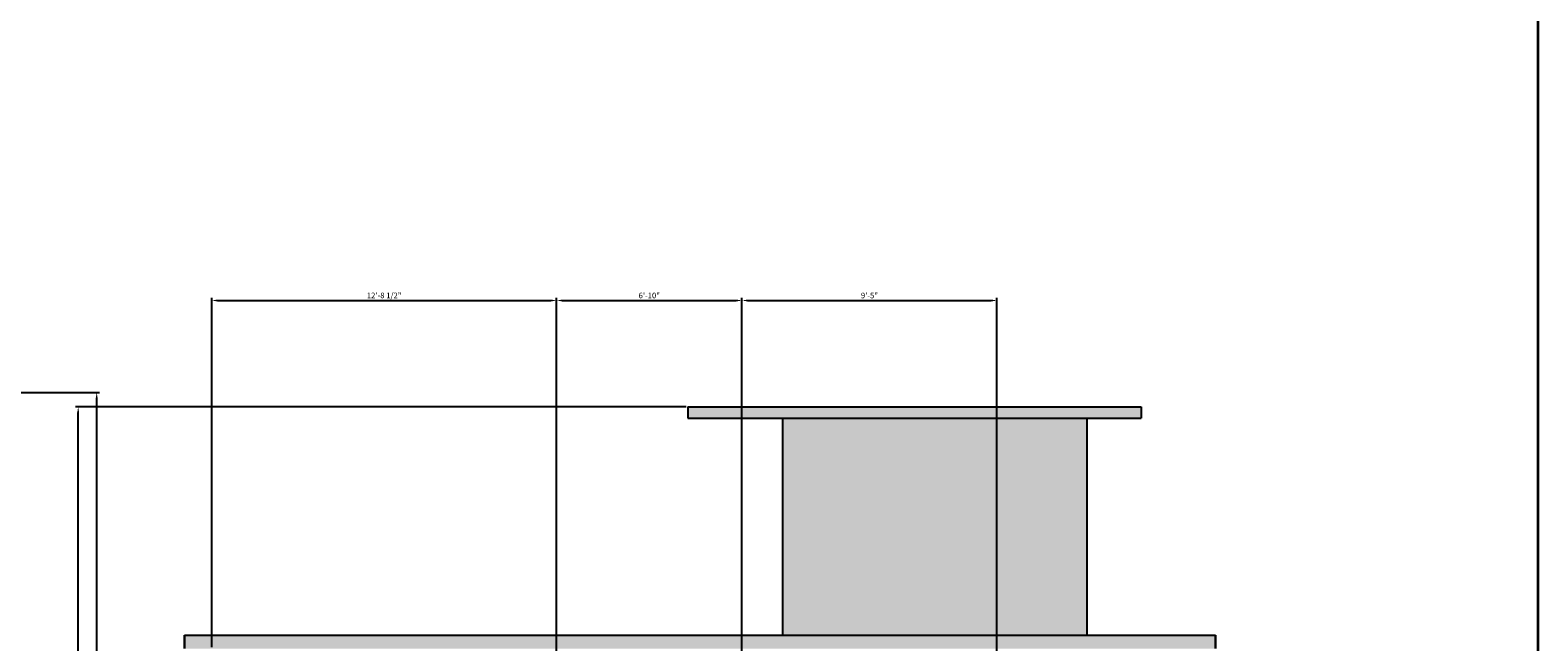
# Model space of a CAD drawing. Units: inches. Extents: x 2391 to 16591, y 7259 to 10239.
# Tile 16 of 27: x 3487 to 4154, y 8229 to 8500. Entities that reach past the tile are written whole.
import ezdxf

# ---------------------------------------------------------------- set-up
doc = ezdxf.new("R2010")
doc.units = ezdxf.units.IN
for name, color, linetype, lineweight in [('A-ANNO-DIMS', 4, 'Continuous', 18), ('A-ANNO-TTLB', 7, 'Continuous', 35), ('A-ELEV', 7, 'Continuous', 30), ('A-ELEV-SURF-PATT', 253, 'Continuous', 13), ('A-ROOF', 7, 'Continuous', 25)]:
    doc.layers.add(name, color=color, linetype=linetype, lineweight=lineweight)
doc.styles.get("Standard").update_dxf_attribs({"font": 'arial.ttf'})
doc.dimstyles.new('ISO-25', dxfattribs={"dimtxt": 2.5, "dimasz": 2.5, "dimexe": 1.25, "dimexo": 0.625, "dimtad": 1, "dimdec": 0, "dimlunit": 3, "dimtxsty": 'Standard', "dimcen": 2.5, "dimadec": 0, "dimazin": 0, "dimtfac": 1, "dimtdec": 0, "dimtmove": 0, "dimatfit": 3, "dimfxl": 1, "dimarcsym": 0})

# ---------------------------------------------------------------- blocks, each defined once
blk = doc.blocks.new('*D84')
at = {"layer": 'A-ANNO-DIMS', "color": 0, "lineweight": -2, "transparency": 16777216}
for p, q in [((3437.4, 8339.52), (3518.08, 8339.52)), ((3516.83, 7579.02), (3516.83, 8337.02)), ((3464.4, 7576.52), (3518.08, 7576.52))]:
    blk.add_line(p, q, dxfattribs=at)
at = {"layer": 'A-ANNO-DIMS', "color": 0, "transparency": 16777216}
for points in [[(3516.41, 8337.02), (3517.24, 8337.02), (3516.83, 8339.52)], [(3516.41, 7579.02), (3517.24, 7579.02), (3516.83, 7576.52)]]:
    blk.add_solid(points, dxfattribs=at)
at = {"layer": 'Defpoints', "color": 0, "transparency": 16777216}
for p in [(3436.78, 8339.52), (3516.83, 8339.52), (3463.78, 7576.52)]:
    blk.add_point(p, dxfattribs=at)
at = {"layer": 'A-ANNO-DIMS', "color": 0, "transparency": 16777216, "insert": (3514.93, 7958.02), "char_height": 2.5, "attachment_point": 5, "rotation": 90}
blk.add_mtext('63\'-7"', dxfattribs=at)
blk = doc.blocks.new('*D92')
at = {"layer": 'A-ANNO-DIMS', "color": 0, "lineweight": -2, "transparency": 16777216}
for p, q in [((3777.58, 8333.18), (3507.41, 8333.18)), ((3508.66, 7572.68), (3508.66, 8330.68)), ((3561.08, 7570.18), (3507.41, 7570.18))]:
    blk.add_line(p, q, dxfattribs=at)
at = {"layer": 'A-ANNO-DIMS', "color": 0, "transparency": 16777216}
for points in [[(3508.24, 8330.68), (3509.08, 8330.68), (3508.66, 8333.18)], [(3508.24, 7572.68), (3509.08, 7572.68), (3508.66, 7570.18)]]:
    blk.add_solid(points, dxfattribs=at)
at = {"layer": 'Defpoints', "color": 0, "transparency": 16777216}
for p in [(3508.66, 8333.18), (3778.21, 8333.18), (3561.71, 7570.18)]:
    blk.add_point(p, dxfattribs=at)
at = {"layer": 'A-ANNO-DIMS', "color": 0, "transparency": 16777216, "insert": (3506.76, 7951.68), "char_height": 2.5, "attachment_point": 5, "rotation": 90}
blk.add_mtext('63\'-7"', dxfattribs=at)
blk = doc.blocks.new('*D93')
at = {"layer": 'A-ANNO-DIMS', "color": 0, "lineweight": -2, "transparency": 16777216}
for p, q in [((3567.71, 8226.81), (3567.71, 8381.48)), ((3570.21, 8380.23), (3717.71, 8380.23)), ((3720.21, 8172.81), (3720.21, 8381.48))]:
    blk.add_line(p, q, dxfattribs=at)
at = {"layer": 'A-ANNO-DIMS', "color": 0, "transparency": 16777216}
for points in [[(3570.21, 8380.65), (3570.21, 8379.81), (3567.71, 8380.23)], [(3717.71, 8380.65), (3717.71, 8379.81), (3720.21, 8380.23)]]:
    blk.add_solid(points, dxfattribs=at)
at = {"layer": 'Defpoints', "color": 0, "transparency": 16777216}
for p in [(3720.21, 8380.23), (3567.71, 8226.18), (3720.21, 8172.18)]:
    blk.add_point(p, dxfattribs=at)
at = {"layer": 'A-ANNO-DIMS', "color": 0, "transparency": 16777216, "insert": (3643.96, 8382.15), "char_height": 2.5, "attachment_point": 5}
blk.add_mtext('12\'-8 1/2"', dxfattribs=at)
blk = doc.blocks.new('*D94')
at = {"layer": 'A-ANNO-DIMS', "color": 0, "lineweight": -2, "transparency": 16777216}
for p, q in [((3720.21, 8172.81), (3720.21, 8381.48)), ((3722.71, 8380.23), (3799.71, 8380.23)), ((3802.21, 8172.81), (3802.21, 8381.48))]:
    blk.add_line(p, q, dxfattribs=at)
at = {"layer": 'A-ANNO-DIMS', "color": 0, "transparency": 16777216}
for points in [[(3722.71, 8380.65), (3722.71, 8379.81), (3720.21, 8380.23)], [(3799.71, 8380.65), (3799.71, 8379.81), (3802.21, 8380.23)]]:
    blk.add_solid(points, dxfattribs=at)
at = {"layer": 'Defpoints', "color": 0, "transparency": 16777216}
for p in [(3802.21, 8380.23), (3720.21, 8172.18), (3802.21, 8172.18)]:
    blk.add_point(p, dxfattribs=at)
at = {"layer": 'A-ANNO-DIMS', "color": 0, "transparency": 16777216, "insert": (3761.21, 8382.13), "char_height": 2.5, "attachment_point": 5}
blk.add_mtext('6\'-10"', dxfattribs=at)
blk = doc.blocks.new('*D95')
at = {"layer": 'A-ANNO-DIMS', "color": 0, "lineweight": -2, "transparency": 16777216}
for p, q in [((3802.21, 8172.81), (3802.21, 8381.48)), ((3804.71, 8380.23), (3912.46, 8380.23)), ((3914.96, 8172.81), (3914.96, 8381.48))]:
    blk.add_line(p, q, dxfattribs=at)
at = {"layer": 'A-ANNO-DIMS', "color": 0, "transparency": 16777216}
for points in [[(3804.71, 8380.65), (3804.71, 8379.81), (3802.21, 8380.23)], [(3912.46, 8380.65), (3912.46, 8379.81), (3914.96, 8380.23)]]:
    blk.add_solid(points, dxfattribs=at)
at = {"layer": 'Defpoints', "color": 0, "transparency": 16777216}
for p in [(3914.96, 8380.23), (3802.21, 8172.18), (3914.96, 8172.18)]:
    blk.add_point(p, dxfattribs=at)
at = {"layer": 'A-ANNO-DIMS', "color": 0, "transparency": 16777216, "insert": (3858.58, 8382.13), "char_height": 2.5, "attachment_point": 5}
blk.add_mtext('9\'-5"', dxfattribs=at)

msp = doc.modelspace()

# ---------------------------------------------------------------- hatches: boundary and pattern name
at = {"layer": 'A-ELEV-SURF-PATT'}
h = msp.add_hatch(color=256, dxfattribs=at)
h.dxf.hatch_style = 1
h.paths.add_polyline_path([(4011.71, 7740.18), (4011.71, 7746.18), (3555.71, 7746.18), (3555.71, 7740.18)])
h.paths.add_polyline_path([(4011.71, 7902.18), (4011.71, 7908.18), (3555.71, 7908.18), (3555.71, 7902.18)])
h.paths.add_polyline_path([(4011.71, 8064.18), (4011.71, 8070.18), (3555.71, 8070.18), (3555.71, 8064.18)])
h.paths.add_polyline_path([(3555.71, 8232.18), (3555.71, 8226.18), (4011.71, 8226.18), (4011.71, 8232.18)])
h.paths.add_polyline_path([(3778.21, 8333.18), (3778.21, 8328.18), (3978.71, 8328.18), (3978.71, 8333.18)])
h = msp.add_hatch(color=256, dxfattribs=at)
h.dxf.hatch_style = 1
h.paths.add_polyline_path([(3954.71, 8328.18), (3820.21, 8328.18), (3820.21, 8232.18), (3954.71, 8232.18)])

# ---------------------------------------------------------------- linework, layer by layer
at = {"layer": 'A-ANNO-TTLB'}
msp.add_lwpolyline([(2391.28, 10239.38), (4154.2, 10239.38), (4154.2, 7258.54), (2391.28, 7258.54)], close=True, dxfattribs=at)
at = {"layer": 'A-ELEV'}
for p, q in [((3555.71, 8226.18), (3555.71, 8232.18)), ((4011.71, 8226.18), (4011.71, 8232.18))]:
    msp.add_line(p, q, dxfattribs=at)
at = {"layer": 'A-ROOF'}
for p, q in [((3778.21, 8333.18), (3978.71, 8333.18)), ((3778.21, 8333.18), (3778.21, 8328.18)), ((3978.71, 8333.18), (3978.71, 8328.18)), ((3778.21, 8328.18), (3978.71, 8328.18)), ((3820.21, 8328.18), (3820.21, 8232.18)), ((3954.71, 8328.18), (3954.71, 8232.18)), ((3555.71, 8232.18), (4011.71, 8232.18))]:
    msp.add_line(p, q, dxfattribs=at)

# ---------------------------------------------------------------- dimensions: what is measured, and where the dimension line sits
at = {"layer": 'A-ANNO-DIMS'}
for base, p1, p2, picture, middle in [((3720.21, 8380.23), (3567.71, 8226.18), (3720.21, 8172.18), '*D93', (3643.96, 8382.15)), ((3802.21, 8380.23), (3720.21, 8172.18), (3802.21, 8172.18), '*D94', (3761.21, 8382.13)), ((3914.959246, 8380.230453), (3802.209246, 8172.180453), (3914.959246, 8172.180453), '*D95', (3858.584246, 8382.13188547))]:
    dim = msp.add_linear_dim(base=base, p1=p1, p2=p2, dimstyle='ISO-25', override={"dimdec": 1, "dimlfac": 1, "dimrnd": 0, "dimzin": 1, "dimdsep": 46, "dimlunit": 4, "dimfrac": 2}, dxfattribs=at)
    dim.commit()
    dim.dimension.update_dxf_attribs({"geometry": picture, "text_midpoint": middle})
for base, p1, p2, picture, middle in [((3516.83, 8339.52), (3463.78, 7576.52), (3436.78, 8339.52), '*D84', (3514.93, 7958.02)), ((3508.66, 8333.18), (3561.71, 7570.18), (3778.21, 8333.18), '*D92', (3506.76, 7951.68))]:
    dim = msp.add_linear_dim(base=base, p1=p1, p2=p2, angle=90, dimstyle='ISO-25', override={"dimdec": 1, "dimlfac": 1, "dimrnd": 0, "dimzin": 1, "dimdsep": 46, "dimlunit": 4, "dimfrac": 2}, dxfattribs=at)
    dim.commit()
    dim.dimension.update_dxf_attribs({"geometry": picture, "text_midpoint": middle})

doc.saveas('drawing.dxf')
